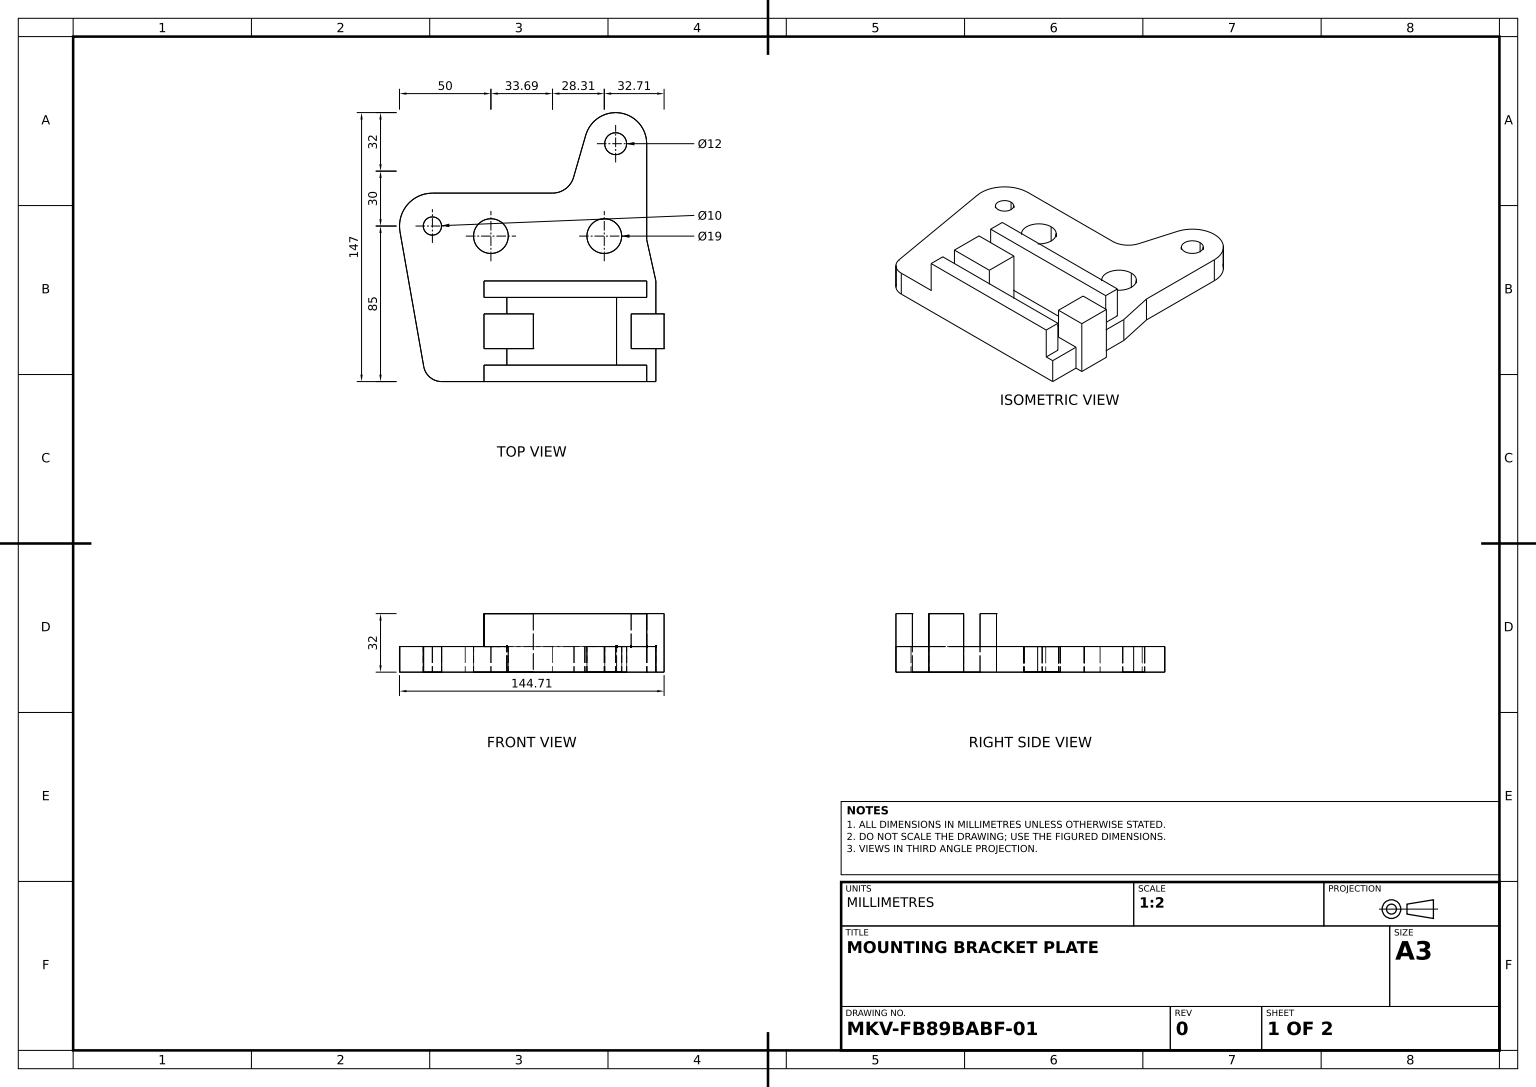
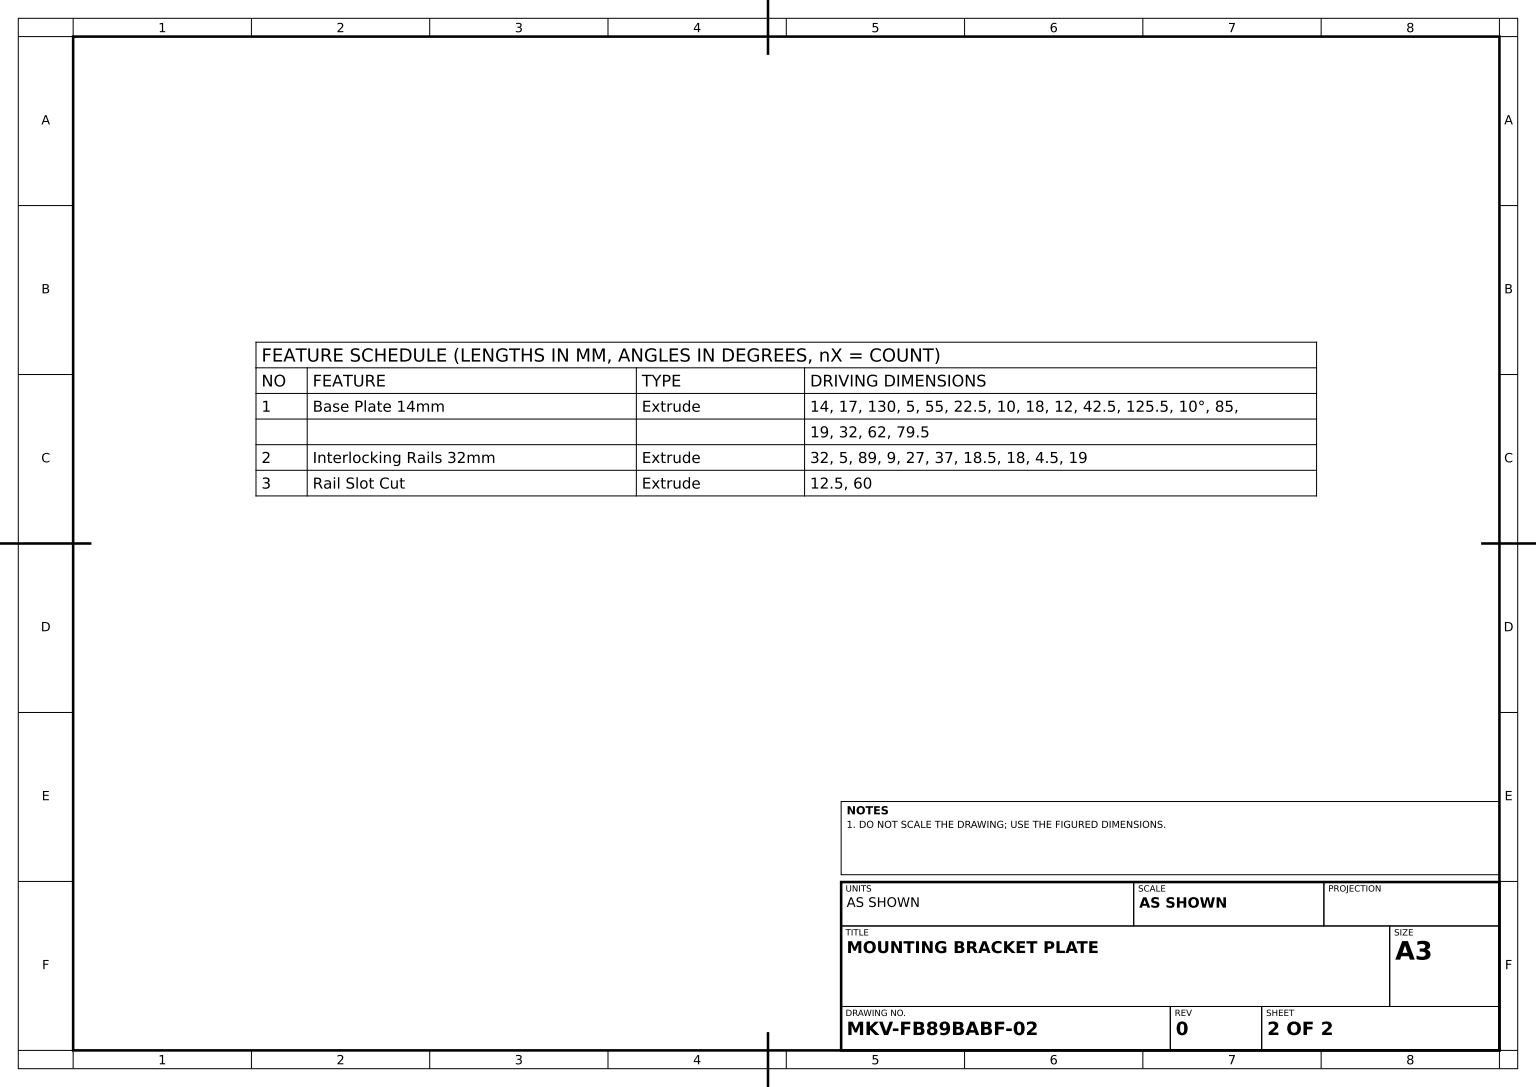
from build123d import *

# Parameters (mm, degrees)
BASE_PLATE_PROFILE_SKETCH_R   = 6
BASE_PLATE_PROFILE_SKETCH_R_2 = 5
BASE_PLATE_PROFILE_SKETCH_R_3 = 9.5
BASE_PLATE_14MM_DEPTH         = 14
INTERLOCKING_RAILS_SKETCH_W   = 89
INTERLOCKING_RAILS_SKETCH_H   = 9
INTERLOCKING_RAILS_SKETCH_W_2 = 27
INTERLOCKING_RAILS_SKETCH_H_2 = 19
INTERLOCKING_RAILS_SKETCH_W_3 = 18
INTERLOCKING_RAILS_32MM_DEPTH = 32
RAIL_SLOT_CUT_REACH           = 205.941


with BuildPart() as part:
    # Base Plate Profile Sketch → Base Plate 14mm (new body)
    with BuildSketch(Plane(origin=(0, 0, 0), x_dir=(1, 0, 0), z_dir=(0, 1, 0))):
        with BuildLine():
            Line((0, 0), (-117.109003688, 0))
            ThreePointArc((-117.109003688, 0), (-123.536879785, 2.339555569), (-126.957081218, 8.263518223))
            Line((-126.957081218, 8.263518223), (-139.9366539, 81.874332802))
            ThreePointArc((-139.9366539, 81.874332802), (-135.998914322, 96.570176974), (-122.210114346, 103))
            Line((-122.210114346, 103), (-56.522720755, 103))
            ThreePointArc((-56.522720755, 103), (-49.311103576, 105.408723877), (-44.994618812, 111.667903721))
            Line((-44.994618812, 111.667903721), (-38.331477751, 134.720469728))
            ThreePointArc((-38.331477751, 134.720469728), (-19.616213283, 146.832039713), (-5, 130))
            Line((-5, 130), (-5, 77.5))
            Line((-5, 77.5), (0, 55))
            Line((0, 55), (0, 0))
        make_face()
        with Locations(Location((-22, 130, 0), (0, 0, 270))):
            Circle(BASE_PLATE_PROFILE_SKETCH_R, mode=Mode.SUBTRACT)
        with Locations(Location((-122.210114346, 85, 0), (0, 0, 270))):
            Circle(BASE_PLATE_PROFILE_SKETCH_R_2, mode=Mode.SUBTRACT)
        with Locations(Location((-90.210114346, 79.5, 0), (0, 0, 270))):
            Circle(BASE_PLATE_PROFILE_SKETCH_R_3, mode=Mode.SUBTRACT)
        with Locations(Location((-28.210114346, 79.5, 0), (0, 0, 270))):
            Circle(BASE_PLATE_PROFILE_SKETCH_R_3, mode=Mode.SUBTRACT)
    extrude(amount=BASE_PLATE_14MM_DEPTH)

    # Interlocking Rails Sketch → Interlocking Rails 32mm (add)
    with BuildSketch(Plane(origin=(0, 0, 0), x_dir=(1, 0, 0), z_dir=(0, 1, 0))):
        with Locations((-49.5, 4.5)):
            Rectangle(INTERLOCKING_RAILS_SKETCH_W, INTERLOCKING_RAILS_SKETCH_H)
        with Locations((-80.5, 27.5)):
            Rectangle(INTERLOCKING_RAILS_SKETCH_W_2, INTERLOCKING_RAILS_SKETCH_H_2)
        with Locations((-49.5, 50.5)):
            Rectangle(INTERLOCKING_RAILS_SKETCH_W, INTERLOCKING_RAILS_SKETCH_H)
        with Locations((-4.5, 27.5)):
            Rectangle(INTERLOCKING_RAILS_SKETCH_W_3, INTERLOCKING_RAILS_SKETCH_H_2)
    extrude(amount=INTERLOCKING_RAILS_32MM_DEPTH)

    # Rail Slot Sketch → Rail Slot Cut (cut, up to next)
    with BuildSketch(Plane(origin=(0, 14, 0), x_dir=(1, 0, 0), z_dir=(0, 1, 0)), mode=Mode.PRIVATE) as rail_slot_cut_sk1:
        Polygon((-81.5, 46), (-81.5, 37), (-67, 37), (-67, 18), (-81.5, 18), (-81.5, 9), (-21.5, 9), (-21.5, 46), align=None)
    rail_slot_cut_tool1 = extrude(rail_slot_cut_sk1.sketch, amount=-RAIL_SLOT_CUT_REACH, mode=Mode.PRIVATE) & part.part
    add(rail_slot_cut_tool1.solids().sort_by_distance((-48.276742, 14, -27.5))[0], mode=Mode.SUBTRACT)


solid = part.part
